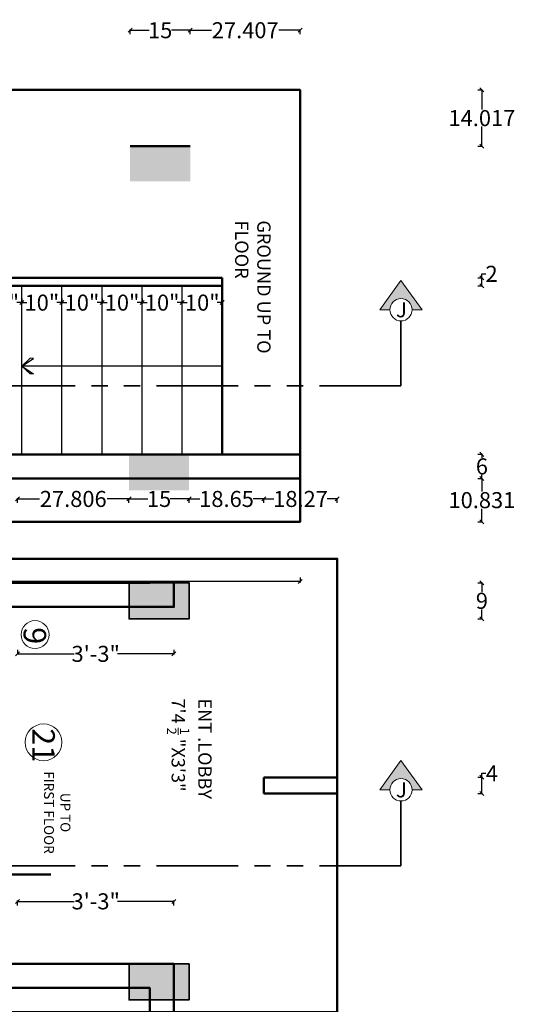
# Model space of a CAD drawing. Units: inches. Extents: x -60 to 284, y -245 to 257.
# Tile 10 of 10: x 160 to 284, y 12 to 257. Entities that reach past the tile are written whole.
import ezdxf

# ---------------------------------------------------------------- set-up
doc = ezdxf.new("R2010")
doc.units = ezdxf.units.IN
doc.header["$LTSCALE"] = 0.8
doc.header["$MEASUREMENT"] = 0
doc.linetypes.add('PHANTOM', pattern=[63.5, 31.75, -6.35, 6.35, -6.35, 6.35, -6.35])
for name, color, linetype, lineweight in [('A-ANNO-DIMS', 2, 'Continuous', 18), ('A-ANNO-SECT', 1, 'PHANTOM', 35), ('A-ANNO-SYMB', 3, 'Continuous', 18), ('A-ANNO-TEXT', 3, 'Continuous', 18), ('A-ANNO-TTLB', 7, 'Continuous', 50), ('A-COLS', 1, 'Continuous', 35), ('A-FLOR-STRS', 4, 'Continuous', 25), ('A-WALL', 7, 'Continuous', 50)]:
    doc.layers.add(name, color=color, linetype=linetype, lineweight=lineweight)
doc.styles.get("Standard").update_dxf_attribs({"font": 'arial.ttf'})
doc.dimstyles.get("Standard").update_dxf_attribs({"dimtxt": 4, "dimasz": 1, "dimexe": 0.18, "dimexo": 0.0625, "dimgap": 0.09, "dimtad": 0, "dimtih": 1, "dimtoh": 1, "dimzin": 0, "dimdsep": 46, "dimlunit": 4, "dimtxsty": 'Standard', "dimblk": 'OBLIQUE', "dimcen": 0.09, "dimadec": 0, "dimazin": 0, "dimtfac": 1, "dimtofl": 0, "dimtmove": 0, "dimatfit": 3, "dimfxl": 1, "dimfxlon": 1, "dimtolj": 1, "dimtzin": 0, "dimarcsym": 0})

# ---------------------------------------------------------------- blocks, each defined once
blk = doc.blocks.new('_Oblique')
at = {"color": 0, "linetype": 'ByBlock', "lineweight": -2}
blk.add_line((-0.5, -0.5), (0.5, 0.5), dxfattribs=at)
blk = doc.blocks.new('*D22')
at = {"layer": 'A-ANNO-DIMS', "color": 0, "lineweight": -2, "ltscale": 0.8, "transparency": 16777216}
for p, q in [((159.94, 36.25), (159.94, 37.43)), ((159.94, 37.25), (174.03, 37.25)), ((198.94, 37.25), (184.84, 37.25)), ((198.94, 36.25), (198.94, 37.43))]:
    blk.add_line(p, q, dxfattribs=at)
at = {"layer": 'Defpoints', "color": 0, "ltscale": 0.8, "transparency": 16777216}
for p in [(198.94, 37.25), (159.94, 21.67), (198.94, 21.67)]:
    blk.add_point(p, dxfattribs=at)
at = {"layer": 'A-ANNO-DIMS', "color": 0, "lineweight": -2, "ltscale": 0.8, "transparency": 16777216, "rotation": 180}
blk.add_blockref('_Oblique', (159.94, 37.25), dxfattribs=at)
at = {"layer": 'A-ANNO-DIMS', "color": 0, "lineweight": -2, "ltscale": 0.8, "transparency": 16777216}
blk.add_blockref('_Oblique', (198.94, 37.25), dxfattribs=at)
at = {"layer": 'A-ANNO-DIMS', "color": 0, "ltscale": 0.8, "transparency": 16777216, "insert": (179.44, 37.25), "char_height": 4, "attachment_point": 5}
blk.add_mtext('\\A1;3\'-3"', dxfattribs=at)
blk = doc.blocks.new('*D23')
at = {"layer": 'A-ANNO-DIMS', "color": 0, "lineweight": -2, "ltscale": 0.8, "transparency": 16777216}
for p, q in [((159.94, 99.95), (159.94, 98.77)), ((159.94, 98.95), (174.03, 98.95)), ((198.94, 98.95), (184.84, 98.95)), ((198.94, 99.95), (198.94, 98.77))]:
    blk.add_line(p, q, dxfattribs=at)
at = {"layer": 'Defpoints', "color": 0, "ltscale": 0.8, "transparency": 16777216}
for p in [(159.94, 110.67), (198.94, 110.67), (198.94, 98.95)]:
    blk.add_point(p, dxfattribs=at)
at = {"layer": 'A-ANNO-DIMS', "color": 0, "lineweight": -2, "ltscale": 0.8, "transparency": 16777216, "rotation": 180}
blk.add_blockref('_Oblique', (159.94, 98.95), dxfattribs=at)
at = {"layer": 'A-ANNO-DIMS', "color": 0, "lineweight": -2, "ltscale": 0.8, "transparency": 16777216}
blk.add_blockref('_Oblique', (198.94, 98.95), dxfattribs=at)
at = {"layer": 'A-ANNO-DIMS', "color": 0, "ltscale": 0.8, "transparency": 16777216, "insert": (179.44, 98.95), "char_height": 4, "attachment_point": 5}
blk.add_mtext('\\A1;3\'-3"', dxfattribs=at)
blk = doc.blocks.new('*D26')
at = {"layer": 'A-ANNO-DIMS', "color": 0, "lineweight": -2, "ltscale": 0.8, "transparency": 16777216}
for p, q in [((201.01, 186.51), (201.01, 186.69)), ((211.01, 186.51), (211.01, 186.69)), ((201.01, 186.51), (202.26, 186.51)), ((211.01, 186.51), (209.77, 186.51))]:
    blk.add_line(p, q, dxfattribs=at)
at = {"layer": 'Defpoints', "color": 0, "ltscale": 0.8, "transparency": 16777216}
for p in [(201.01, 186.51), (201.01, 186.51), (211.01, 186.51)]:
    blk.add_point(p, dxfattribs=at)
at = {"layer": 'A-ANNO-DIMS', "color": 0, "lineweight": -2, "ltscale": 0.8, "transparency": 16777216, "rotation": 180}
blk.add_blockref('_Oblique', (201.01, 186.51), dxfattribs=at)
at = {"layer": 'A-ANNO-DIMS', "color": 0, "lineweight": -2, "ltscale": 0.8, "transparency": 16777216}
blk.add_blockref('_Oblique', (211.01, 186.51), dxfattribs=at)
at = {"layer": 'A-ANNO-DIMS', "color": 0, "ltscale": 0.8, "transparency": 16777216, "insert": (206.01, 186.51), "char_height": 4, "attachment_point": 5}
blk.add_mtext('\\A1;10"', dxfattribs=at)
blk = doc.blocks.new('*D27')
at = {"layer": 'A-ANNO-DIMS', "color": 0, "lineweight": -2, "ltscale": 0.8, "transparency": 16777216}
for p, q in [((191.01, 186.51), (191.01, 186.69)), ((201.01, 186.51), (201.01, 186.69)), ((191.01, 186.51), (192.26, 186.51)), ((201.01, 186.51), (199.77, 186.51))]:
    blk.add_line(p, q, dxfattribs=at)
at = {"layer": 'Defpoints', "color": 0, "ltscale": 0.8, "transparency": 16777216}
for p in [(191.01, 186.51), (191.01, 186.51), (201.01, 186.51)]:
    blk.add_point(p, dxfattribs=at)
at = {"layer": 'A-ANNO-DIMS', "color": 0, "lineweight": -2, "ltscale": 0.8, "transparency": 16777216, "rotation": 180}
blk.add_blockref('_Oblique', (191.01, 186.51), dxfattribs=at)
at = {"layer": 'A-ANNO-DIMS', "color": 0, "lineweight": -2, "ltscale": 0.8, "transparency": 16777216}
blk.add_blockref('_Oblique', (201.01, 186.51), dxfattribs=at)
at = {"layer": 'A-ANNO-DIMS', "color": 0, "ltscale": 0.8, "transparency": 16777216, "insert": (196.01, 186.51), "char_height": 4, "attachment_point": 5}
blk.add_mtext('\\A1;10"', dxfattribs=at)
blk = doc.blocks.new('*D28')
at = {"layer": 'A-ANNO-DIMS', "color": 0, "lineweight": -2, "ltscale": 0.8, "transparency": 16777216}
for p, q in [((181.01, 187.51), (181.01, 186.33)), ((191.01, 187.51), (191.01, 186.33)), ((181.01, 186.51), (182.26, 186.51)), ((191.01, 186.51), (189.77, 186.51))]:
    blk.add_line(p, q, dxfattribs=at)
at = {"layer": 'Defpoints', "color": 0, "ltscale": 0.8, "transparency": 16777216}
for p in [(181.01, 187.62), (191.01, 187.62), (191.01, 186.51)]:
    blk.add_point(p, dxfattribs=at)
at = {"layer": 'A-ANNO-DIMS', "color": 0, "lineweight": -2, "ltscale": 0.8, "transparency": 16777216, "rotation": 180}
blk.add_blockref('_Oblique', (181.01, 186.51), dxfattribs=at)
at = {"layer": 'A-ANNO-DIMS', "color": 0, "lineweight": -2, "ltscale": 0.8, "transparency": 16777216}
blk.add_blockref('_Oblique', (191.01, 186.51), dxfattribs=at)
at = {"layer": 'A-ANNO-DIMS', "color": 0, "ltscale": 0.8, "transparency": 16777216, "insert": (186.01, 186.51), "char_height": 4, "attachment_point": 5}
blk.add_mtext('\\A1;10"', dxfattribs=at)
blk = doc.blocks.new('*D29')
at = {"layer": 'A-ANNO-DIMS', "color": 0, "lineweight": -2, "ltscale": 0.8, "transparency": 16777216}
for p, q in [((171.01, 187.47), (171.01, 186.33)), ((181.01, 187.51), (181.01, 186.33)), ((171.01, 186.51), (172.26, 186.51)), ((181.01, 186.51), (179.77, 186.51))]:
    blk.add_line(p, q, dxfattribs=at)
at = {"layer": 'Defpoints', "color": 0, "ltscale": 0.8, "transparency": 16777216}
for p in [(171.01, 187.53), (181.01, 187.62), (181.01, 186.51)]:
    blk.add_point(p, dxfattribs=at)
at = {"layer": 'A-ANNO-DIMS', "color": 0, "lineweight": -2, "ltscale": 0.8, "transparency": 16777216, "rotation": 180}
blk.add_blockref('_Oblique', (171.01, 186.51), dxfattribs=at)
at = {"layer": 'A-ANNO-DIMS', "color": 0, "lineweight": -2, "ltscale": 0.8, "transparency": 16777216}
blk.add_blockref('_Oblique', (181.01, 186.51), dxfattribs=at)
at = {"layer": 'A-ANNO-DIMS', "color": 0, "ltscale": 0.8, "transparency": 16777216, "insert": (176.01, 186.51), "char_height": 4, "attachment_point": 5}
blk.add_mtext('\\A1;10"', dxfattribs=at)
blk = doc.blocks.new('*D30')
at = {"layer": 'A-ANNO-DIMS', "color": 0, "lineweight": -2, "ltscale": 0.8, "transparency": 16777216}
for p, q in [((161.01, 187.51), (161.01, 186.33)), ((171.01, 187.51), (171.01, 186.33)), ((161.01, 186.51), (162.26, 186.51)), ((171.01, 186.51), (169.77, 186.51))]:
    blk.add_line(p, q, dxfattribs=at)
at = {"layer": 'Defpoints', "color": 0, "ltscale": 0.8, "transparency": 16777216}
for p in [(161.01, 187.69), (171.01, 187.69), (171.01, 186.51)]:
    blk.add_point(p, dxfattribs=at)
at = {"layer": 'A-ANNO-DIMS', "color": 0, "lineweight": -2, "ltscale": 0.8, "transparency": 16777216, "rotation": 180}
blk.add_blockref('_Oblique', (161.01, 186.51), dxfattribs=at)
at = {"layer": 'A-ANNO-DIMS', "color": 0, "lineweight": -2, "ltscale": 0.8, "transparency": 16777216}
blk.add_blockref('_Oblique', (171.01, 186.51), dxfattribs=at)
at = {"layer": 'A-ANNO-DIMS', "color": 0, "ltscale": 0.8, "transparency": 16777216, "insert": (166.01, 186.51), "char_height": 4, "attachment_point": 5}
blk.add_mtext('\\A1;10"', dxfattribs=at)
blk = doc.blocks.new('*D31')
at = {"layer": 'A-ANNO-DIMS', "color": 0, "lineweight": -2, "ltscale": 0.8, "transparency": 16777216}
for p, q in [((151.01, 187.51), (151.01, 186.33)), ((161.01, 187.51), (161.01, 186.33)), ((151.01, 186.51), (152.26, 186.51)), ((161.01, 186.51), (159.77, 186.51))]:
    blk.add_line(p, q, dxfattribs=at)
at = {"layer": 'Defpoints', "color": 0, "ltscale": 0.8, "transparency": 16777216}
for p in [(151.01, 187.73), (161.01, 187.73), (161.01, 186.51)]:
    blk.add_point(p, dxfattribs=at)
at = {"layer": 'A-ANNO-DIMS', "color": 0, "lineweight": -2, "ltscale": 0.8, "transparency": 16777216, "rotation": 180}
blk.add_blockref('_Oblique', (151.01, 186.51), dxfattribs=at)
at = {"layer": 'A-ANNO-DIMS', "color": 0, "lineweight": -2, "ltscale": 0.8, "transparency": 16777216}
blk.add_blockref('_Oblique', (161.01, 186.51), dxfattribs=at)
at = {"layer": 'A-ANNO-DIMS', "color": 0, "ltscale": 0.8, "transparency": 16777216, "insert": (156.01, 186.51), "char_height": 4, "attachment_point": 5}
blk.add_mtext('\\A1;10"', dxfattribs=at)
blk = doc.blocks.new('SECTION-MARK')
at = {"ltscale": 0.8}
for p, q in [((0, 2.79), (5.28, 10.08)), ((10.57, 2.79), (5.28, 10.08)), ((2.5, 2.79), (0, 2.79)), ((8.07, 2.79), (10.57, 2.79))]:
    blk.add_line(p, q, dxfattribs=at)
blk.add_circle((5.28, 2.79), 2.79, dxfattribs=at)
blk = doc.blocks.new('STAIR-ARROW')
at = {"ltscale": 0.8}
for p, q in [((2.04, 3.88), (0, 1.94)), ((0, 1.94), (2.88, 3.86)), ((2.88, 3.86), (2.04, 3.88)), ((50, 1.94), (0, 1.94)), ((0, 1.94), (2.88, 0.03)), ((2.04, 0), (0, 1.94)), ((2.88, 0.03), (2.04, 0))]:
    blk.add_line(p, q, dxfattribs=at)
blk = doc.blocks.new('*D76')
at = {"layer": 'A-ANNO-DIMS', "color": 0, "lineweight": -2, "ltscale": 0.8, "transparency": 16777216}
for p, q in [((-0.88, 117.95), (-0.88, 116.77)), ((230.43, 117.95), (230.43, 116.77)), ((-0.88, 116.95), (107.9, 116.95)), ((230.43, 116.95), (121.65, 116.95))]:
    blk.add_line(p, q, dxfattribs=at)
at = {"layer": 'Defpoints', "color": 0, "ltscale": 0.8, "transparency": 16777216}
for p in [(-0.88, 131.85), (230.43, 131.85), (230.43, 116.95)]:
    blk.add_point(p, dxfattribs=at)
at = {"layer": 'A-ANNO-DIMS', "color": 0, "lineweight": -2, "ltscale": 0.8, "transparency": 16777216, "rotation": 180}
blk.add_blockref('_Oblique', (-0.88, 116.95), dxfattribs=at)
at = {"layer": 'A-ANNO-DIMS', "color": 0, "lineweight": -2, "ltscale": 0.8, "transparency": 16777216}
blk.add_blockref('_Oblique', (230.43, 116.95), dxfattribs=at)
at = {"layer": 'A-ANNO-DIMS', "color": 0, "ltscale": 0.8, "transparency": 16777216, "insert": (114.78, 116.95), "char_height": 4, "attachment_point": 5}
blk.add_mtext('\\A1;231.3', dxfattribs=at)
blk = doc.blocks.new('*D81')
at = {"layer": 'A-ANNO-DIMS', "color": 0, "lineweight": -2, "ltscale": 0.8, "transparency": 16777216}
for p, q in [((188.02, 253.42), (188.02, 254.6)), ((188.02, 254.42), (192.74, 254.42)), ((203.02, 254.42), (198.3, 254.42)), ((203.02, 253.42), (203.02, 254.6))]:
    blk.add_line(p, q, dxfattribs=at)
at = {"layer": 'Defpoints', "color": 0, "ltscale": 0.8, "transparency": 16777216}
for p in [(203.02, 254.42), (188.02, 225.5), (203.02, 225.5)]:
    blk.add_point(p, dxfattribs=at)
at = {"layer": 'A-ANNO-DIMS', "color": 0, "lineweight": -2, "ltscale": 0.8, "transparency": 16777216, "rotation": 180}
blk.add_blockref('_Oblique', (188.02, 254.42), dxfattribs=at)
at = {"layer": 'A-ANNO-DIMS', "color": 0, "lineweight": -2, "ltscale": 0.8, "transparency": 16777216}
blk.add_blockref('_Oblique', (203.02, 254.42), dxfattribs=at)
at = {"layer": 'A-ANNO-DIMS', "color": 0, "ltscale": 0.8, "transparency": 16777216, "insert": (195.52, 254.42), "char_height": 4, "attachment_point": 5}
blk.add_mtext('\\A1;15', dxfattribs=at)
blk = doc.blocks.new('*D82')
at = {"layer": 'A-ANNO-DIMS', "color": 0, "lineweight": -2, "ltscale": 0.8, "transparency": 16777216}
for p, q in [((203.02, 253.42), (203.02, 254.6)), ((203.02, 254.42), (208.3, 254.42)), ((230.43, 254.42), (225.15, 254.42)), ((230.43, 253.42), (230.43, 254.6))]:
    blk.add_line(p, q, dxfattribs=at)
at = {"layer": 'Defpoints', "color": 0, "ltscale": 0.8, "transparency": 16777216}
for p in [(230.43, 254.42), (230.43, 239.52), (203.02, 225.5)]:
    blk.add_point(p, dxfattribs=at)
at = {"layer": 'A-ANNO-DIMS', "color": 0, "lineweight": -2, "ltscale": 0.8, "transparency": 16777216, "rotation": 180}
blk.add_blockref('_Oblique', (203.02, 254.42), dxfattribs=at)
at = {"layer": 'A-ANNO-DIMS', "color": 0, "lineweight": -2, "ltscale": 0.8, "transparency": 16777216}
blk.add_blockref('_Oblique', (230.43, 254.42), dxfattribs=at)
at = {"layer": 'A-ANNO-DIMS', "color": 0, "ltscale": 0.8, "transparency": 16777216, "insert": (216.73, 254.42), "char_height": 4, "attachment_point": 5}
blk.add_mtext('\\A1;27.407', dxfattribs=at)
blk = doc.blocks.new('*D83')
at = {"layer": 'A-ANNO-DIMS', "color": 0, "lineweight": -2, "ltscale": 0.8, "transparency": 16777216}
for p, q in [((274.76, 148.69), (275.94, 148.69)), ((275.76, 148.69), (275.76, 147.82)), ((274.76, 142.69), (275.94, 142.69)), ((275.76, 142.69), (275.76, 143.55))]:
    blk.add_line(p, q, dxfattribs=at)
at = {"layer": 'Defpoints', "color": 0, "ltscale": 0.8, "transparency": 16777216}
for p in [(230.43, 148.69), (275.76, 148.69), (230.43, 142.69)]:
    blk.add_point(p, dxfattribs=at)
at = {"layer": 'A-ANNO-DIMS', "color": 0, "lineweight": -2, "ltscale": 0.8, "transparency": 16777216}
for p, rotation in [((275.76, 148.69), 90), ((275.76, 142.69), 270)]:
    blk.add_blockref('_Oblique', p, dxfattribs=dict(at, rotation=rotation))
at = {"layer": 'A-ANNO-DIMS', "color": 0, "ltscale": 0.8, "transparency": 16777216, "insert": (275.76, 145.69), "char_height": 4, "attachment_point": 5}
blk.add_mtext('\\A1;6', dxfattribs=at)
blk = doc.blocks.new('*D84')
at = {"layer": 'A-ANNO-DIMS', "color": 0, "lineweight": -2, "ltscale": 0.8, "transparency": 16777216}
for p, q in [((274.76, 142.69), (275.94, 142.69)), ((275.76, 142.69), (275.76, 139.4)), ((275.76, 131.85), (275.76, 135.14)), ((274.76, 131.85), (275.94, 131.85))]:
    blk.add_line(p, q, dxfattribs=at)
at = {"layer": 'Defpoints', "color": 0, "ltscale": 0.8, "transparency": 16777216}
for p in [(230.43, 142.69), (275.76, 142.69), (230.43, 131.85)]:
    blk.add_point(p, dxfattribs=at)
at = {"layer": 'A-ANNO-DIMS', "color": 0, "lineweight": -2, "ltscale": 0.8, "transparency": 16777216}
for p, rotation in [((275.76, 142.69), 90), ((275.76, 131.85), 270)]:
    blk.add_blockref('_Oblique', p, dxfattribs=dict(at, rotation=rotation))
at = {"layer": 'A-ANNO-DIMS', "color": 0, "ltscale": 0.8, "transparency": 16777216, "insert": (275.76, 137.27), "char_height": 4, "attachment_point": 5}
blk.add_mtext('\\A1;10.831', dxfattribs=at)
blk = doc.blocks.new('*D85')
at = {"layer": 'A-ANNO-DIMS', "color": 0, "lineweight": -2, "ltscale": 0.8, "transparency": 16777216}
for p, q in [((274.76, 192.69), (275.94, 192.69)), ((275.76, 192.69), (275.76, 193.69)), ((275.76, 193.69), (276.76, 193.69)), ((275.76, 190.69), (275.76, 192.69)), ((274.76, 190.69), (275.94, 190.69))]:
    blk.add_line(p, q, dxfattribs=at)
at = {"layer": 'Defpoints', "color": 0, "ltscale": 0.8, "transparency": 16777216}
for p in [(211.01, 192.69), (275.76, 192.69), (211.01, 190.69)]:
    blk.add_point(p, dxfattribs=at)
at = {"layer": 'A-ANNO-DIMS', "color": 0, "lineweight": -2, "ltscale": 0.8, "transparency": 16777216}
for p, rotation in [((275.76, 192.69), 90), ((275.76, 190.69), 270)]:
    blk.add_blockref('_Oblique', p, dxfattribs=dict(at, rotation=rotation))
at = {"layer": 'A-ANNO-DIMS', "color": 0, "ltscale": 0.8, "transparency": 16777216, "insert": (278.18, 193.69), "char_height": 4, "attachment_point": 5}
blk.add_mtext('\\A1;2', dxfattribs=at)
blk = doc.blocks.new('*D86')
at = {"layer": 'A-ANNO-DIMS', "color": 0, "lineweight": -2, "ltscale": 0.8, "transparency": 16777216}
for p, q in [((274.76, 239.52), (275.94, 239.52)), ((275.76, 239.52), (275.76, 234.64)), ((275.76, 225.5), (275.76, 230.38)), ((274.76, 225.5), (275.94, 225.5))]:
    blk.add_line(p, q, dxfattribs=at)
at = {"layer": 'Defpoints', "color": 0, "ltscale": 0.8, "transparency": 16777216}
for p in [(230.43, 239.52), (275.76, 239.52), (203.02, 225.5)]:
    blk.add_point(p, dxfattribs=at)
at = {"layer": 'A-ANNO-DIMS', "color": 0, "lineweight": -2, "ltscale": 0.8, "transparency": 16777216}
for p, rotation in [((275.76, 239.52), 90), ((275.76, 225.5), 270)]:
    blk.add_blockref('_Oblique', p, dxfattribs=dict(at, rotation=rotation))
at = {"layer": 'A-ANNO-DIMS', "color": 0, "ltscale": 0.8, "transparency": 16777216, "insert": (275.76, 232.51), "char_height": 4, "attachment_point": 5}
blk.add_mtext('\\A1;14.017', dxfattribs=at)
blk = doc.blocks.new('*D95')
at = {"layer": 'A-ANNO-DIMS', "color": 0, "lineweight": -2, "ltscale": 0.8, "transparency": 16777216}
for p, q in [((159.94, 136.57), (159.94, 137.75)), ((159.94, 137.57), (165.41, 137.57)), ((187.74, 137.57), (182.26, 137.57)), ((187.74, 136.57), (187.74, 137.75))]:
    blk.add_line(p, q, dxfattribs=at)
at = {"layer": 'Defpoints', "color": 0, "ltscale": 0.8, "transparency": 16777216}
for p in [(187.74, 137.57), (159.94, 110.67), (187.74, 107.67)]:
    blk.add_point(p, dxfattribs=at)
at = {"layer": 'A-ANNO-DIMS', "color": 0, "lineweight": -2, "ltscale": 0.8, "transparency": 16777216, "rotation": 180}
blk.add_blockref('_Oblique', (159.94, 137.57), dxfattribs=at)
at = {"layer": 'A-ANNO-DIMS', "color": 0, "lineweight": -2, "ltscale": 0.8, "transparency": 16777216}
blk.add_blockref('_Oblique', (187.74, 137.57), dxfattribs=at)
at = {"layer": 'A-ANNO-DIMS', "color": 0, "ltscale": 0.8, "transparency": 16777216, "insert": (173.84, 137.57), "char_height": 4, "attachment_point": 5}
blk.add_mtext('\\A1;27.806', dxfattribs=at)
blk = doc.blocks.new('*D96')
at = {"layer": 'A-ANNO-DIMS', "color": 0, "lineweight": -2, "ltscale": 0.8, "transparency": 16777216}
for p, q in [((187.74, 136.57), (187.74, 137.75)), ((187.74, 137.57), (192.46, 137.57)), ((202.74, 137.57), (198.02, 137.57)), ((202.74, 136.57), (202.74, 137.75))]:
    blk.add_line(p, q, dxfattribs=at)
at = {"layer": 'Defpoints', "color": 0, "ltscale": 0.8, "transparency": 16777216}
for p in [(202.74, 137.57), (187.74, 107.67), (202.74, 107.67)]:
    blk.add_point(p, dxfattribs=at)
at = {"layer": 'A-ANNO-DIMS', "color": 0, "lineweight": -2, "ltscale": 0.8, "transparency": 16777216, "rotation": 180}
blk.add_blockref('_Oblique', (187.74, 137.57), dxfattribs=at)
at = {"layer": 'A-ANNO-DIMS', "color": 0, "lineweight": -2, "ltscale": 0.8, "transparency": 16777216}
blk.add_blockref('_Oblique', (202.74, 137.57), dxfattribs=at)
at = {"layer": 'A-ANNO-DIMS', "color": 0, "ltscale": 0.8, "transparency": 16777216, "insert": (195.24, 137.57), "char_height": 4, "attachment_point": 5}
blk.add_mtext('\\A1;15', dxfattribs=at)
blk = doc.blocks.new('*D97')
at = {"layer": 'A-ANNO-DIMS', "color": 0, "lineweight": -2, "ltscale": 0.8, "transparency": 16777216}
for p, q in [((202.74, 136.57), (202.74, 137.75)), ((202.74, 137.57), (205.4, 137.57)), ((221.39, 137.57), (218.73, 137.57)), ((221.39, 136.57), (221.39, 137.75))]:
    blk.add_line(p, q, dxfattribs=at)
at = {"layer": 'Defpoints', "color": 0, "ltscale": 0.8, "transparency": 16777216}
for p in [(221.39, 137.57), (202.74, 107.67), (221.39, 68.17)]:
    blk.add_point(p, dxfattribs=at)
at = {"layer": 'A-ANNO-DIMS', "color": 0, "lineweight": -2, "ltscale": 0.8, "transparency": 16777216, "rotation": 180}
blk.add_blockref('_Oblique', (202.74, 137.57), dxfattribs=at)
at = {"layer": 'A-ANNO-DIMS', "color": 0, "lineweight": -2, "ltscale": 0.8, "transparency": 16777216}
blk.add_blockref('_Oblique', (221.39, 137.57), dxfattribs=at)
at = {"layer": 'A-ANNO-DIMS', "color": 0, "ltscale": 0.8, "transparency": 16777216, "insert": (212.07, 137.57), "char_height": 4, "attachment_point": 5}
blk.add_mtext('\\A1;18.65', dxfattribs=at)
blk = doc.blocks.new('*D98')
at = {"layer": 'A-ANNO-DIMS', "color": 0, "lineweight": -2, "ltscale": 0.8, "transparency": 16777216}
for p, q in [((221.39, 136.57), (221.39, 137.75)), ((221.39, 137.57), (223.88, 137.57)), ((239.66, 137.57), (237.18, 137.57)), ((239.66, 136.57), (239.66, 137.75))]:
    blk.add_line(p, q, dxfattribs=at)
at = {"layer": 'Defpoints', "color": 0, "ltscale": 0.8, "transparency": 16777216}
for p in [(239.66, 137.57), (239.66, 122.67), (221.39, 68.17)]:
    blk.add_point(p, dxfattribs=at)
at = {"layer": 'A-ANNO-DIMS', "color": 0, "lineweight": -2, "ltscale": 0.8, "transparency": 16777216, "rotation": 180}
blk.add_blockref('_Oblique', (221.39, 137.57), dxfattribs=at)
at = {"layer": 'A-ANNO-DIMS', "color": 0, "lineweight": -2, "ltscale": 0.8, "transparency": 16777216}
blk.add_blockref('_Oblique', (239.66, 137.57), dxfattribs=at)
at = {"layer": 'A-ANNO-DIMS', "color": 0, "ltscale": 0.8, "transparency": 16777216, "insert": (230.53, 137.57), "char_height": 4, "attachment_point": 5}
blk.add_mtext('\\A1;18.27', dxfattribs=at)
blk = doc.blocks.new('*D103')
at = {"layer": 'A-ANNO-DIMS', "color": 0, "lineweight": -2, "ltscale": 0.8, "transparency": 16777216}
for p, q in [((274.76, 116.67), (275.94, 116.67)), ((275.76, 116.67), (275.76, 114.3)), ((275.76, 107.67), (275.76, 110.03)), ((274.76, 107.67), (275.94, 107.67))]:
    blk.add_line(p, q, dxfattribs=at)
at = {"layer": 'Defpoints', "color": 0, "ltscale": 0.8, "transparency": 16777216}
for p in [(202.74, 116.67), (275.76, 116.67), (202.74, 107.67)]:
    blk.add_point(p, dxfattribs=at)
at = {"layer": 'A-ANNO-DIMS', "color": 0, "lineweight": -2, "ltscale": 0.8, "transparency": 16777216}
for p, rotation in [((275.76, 116.67), 90), ((275.76, 107.67), 270)]:
    blk.add_blockref('_Oblique', p, dxfattribs=dict(at, rotation=rotation))
at = {"layer": 'A-ANNO-DIMS', "color": 0, "ltscale": 0.8, "transparency": 16777216, "insert": (275.76, 112.17), "char_height": 4, "attachment_point": 5}
blk.add_mtext('\\A1;9', dxfattribs=at)
blk = doc.blocks.new('*D104')
at = {"layer": 'A-ANNO-DIMS', "color": 0, "lineweight": -2, "ltscale": 0.8, "transparency": 16777216}
for p, q in [((275.76, 68.17), (275.76, 69.17)), ((275.76, 69.17), (276.76, 69.17)), ((274.76, 68.17), (275.94, 68.17)), ((275.76, 64.17), (275.76, 68.17)), ((274.76, 64.17), (275.94, 64.17))]:
    blk.add_line(p, q, dxfattribs=at)
at = {"layer": 'Defpoints', "color": 0, "ltscale": 0.8, "transparency": 16777216}
for p in [(221.39, 68.17), (275.76, 68.17), (221.39, 64.17)]:
    blk.add_point(p, dxfattribs=at)
at = {"layer": 'A-ANNO-DIMS', "color": 0, "lineweight": -2, "ltscale": 0.8, "transparency": 16777216}
for p, rotation in [((275.76, 68.17), 90), ((275.76, 64.17), 270)]:
    blk.add_blockref('_Oblique', p, dxfattribs=dict(at, rotation=rotation))
at = {"layer": 'A-ANNO-DIMS', "color": 0, "ltscale": 0.8, "transparency": 16777216, "insert": (278.24, 69.17), "char_height": 4, "attachment_point": 5}
blk.add_mtext('\\A1;4', dxfattribs=at)

msp = doc.modelspace()

# ---------------------------------------------------------------- hatches: boundary and pattern name
at = {"layer": 'A-ANNO-SYMB', "ltscale": 0.8}
h = msp.add_hatch(color=256, dxfattribs=at)
h.dxf.hatch_style = 1
h.paths.add_polyline_path([(250.2979, 184.7402), (252.7949, 184.7402, -1), (258.3665, 184.7402), (260.8636, 184.7402), (255.5807, 192.0356)])
h = msp.add_hatch(color=256, dxfattribs=at)
h.dxf.hatch_style = 1
h.paths.add_polyline_path([(255.5807, 72.3512), (250.2979, 65.0558), (252.7949, 65.0558, -1), (258.3665, 65.0558), (260.8636, 65.0558)])
at = {"layer": 'A-COLS', "ltscale": 0.8}
h = msp.add_hatch(color=256, dxfattribs=at)
h.dxf.hatch_style = 1
h.paths.add_polyline_path([(203.0229, 225.7452), (188.0229, 225.7452), (188.0229, 216.7452), (203.0229, 216.7452)])
h = msp.add_hatch(color=256, dxfattribs=at)
h.dxf.hatch_style = 1
h.paths.add_polyline_path([(202.7426, 148.6856), (187.7426, 148.6856), (187.7426, 139.6856), (202.7426, 139.6856)])
h = msp.add_hatch(color=256, dxfattribs=at)
h.dxf.hatch_style = 1
h.paths.add_polyline_path([(202.7426, 116.666), (187.7426, 116.666), (187.7426, 107.666), (202.7426, 107.666)])
h = msp.add_hatch(color=256, dxfattribs=at)
h.dxf.hatch_style = 1
h.paths.add_polyline_path([(202.7426, 21.666), (187.7426, 21.666), (187.7426, 12.666), (202.7426, 12.666)])

# ---------------------------------------------------------------- linework, layer by layer
at = {"layer": 'A-ANNO-SECT', "ltscale": 0.8}
for p, q in [((255.5807, 181.9544), (255.5807, 165.8004)), ((255.5807, 165.8004), (-23.5489, 165.8004)), ((255.5807, 62.27), (255.5807, 46.116)), ((255.5807, 46.116), (-23.5489, 46.116))]:
    msp.add_line(p, q, dxfattribs=at)
at = {"layer": 'A-ANNO-SYMB', "ltscale": 0.8}
for centre, radius in [((164.3195, 103.7534), 3.4808), ((166.4188, 76.8954), 4.5856)]:
    msp.add_circle(centre, radius, dxfattribs=at)
at = {"layer": 'A-ANNO-TTLB', "ltscale": 0.8}
for points in [[(-0.8787, 239.5184), (230.4297, 239.5184), (230.4297, 131.8542), (-0.8787, 131.8542)], [(0.0867, 122.666), (239.6639, 122.666), (239.6639, 9.666), (0.0867, 9.666)]]:
    msp.add_lwpolyline(points, close=True, dxfattribs=at)
at = {"layer": 'A-COLS', "ltscale": 0.8}
for points in [[(187.7426, 116.666), (202.7426, 116.666), (202.7426, 107.666), (187.7426, 107.666)], [(187.7426, 21.666), (202.7426, 21.666), (202.7426, 12.666), (187.7426, 12.666)]]:
    msp.add_lwpolyline(points, close=True, dxfattribs=at)
at = {"layer": 'A-FLOR-STRS', "ltscale": 0.8}
for p, q in [((161.0139, 148.6856), (161.0139, 190.6856)), ((171.0139, 148.6856), (171.0139, 190.6856)), ((181.0139, 148.6856), (181.0139, 190.6856)), ((191.0139, 148.6856), (191.0139, 190.6856)), ((201.0139, 148.6856), (201.0139, 190.6856))]:
    msp.add_line(p, q, dxfattribs=at)
at = {"layer": 'A-WALL', "ltscale": 0.8}
for p, q in [((203.0229, 225.5014), (188.0229, 225.5014)), ((67.0139, 192.6856), (211.0139, 192.6856)), ((211.0139, 148.6856), (211.0139, 192.6856)), ((67.0139, 190.6856), (211.0139, 190.6856)), ((82.0139, 148.6856), (230.4297, 148.6856)), ((82.0139, 142.6856), (230.4297, 142.6856)), ((239.6639, 68.166), (221.3929, 68.166)), ((221.3929, 64.166), (221.3929, 68.166)), ((239.6639, 64.166), (221.3929, 64.166)), ((168.271, 43.916), (43.6123, 43.916))]:
    msp.add_line(p, q, dxfattribs=at)
at = {"layer": 'A-WALL'}
for points in [[(198.9361, 116.666), (198.9361, 110.666), (159.9361, 110.666), (79.9361, 110.666), (37.9361, 110.666), (27.9361, 110.666), (27.9361, 122.666)], [(192.9361, 116.666), (159.9361, 116.666), (79.9361, 116.666), (37.9361, 116.666), (33.9361, 116.666), (33.9361, 122.666)], [(198.9361, 9.666), (198.9361, 21.666), (159.9361, 21.666), (79.9361, 21.666), (37.9361, 21.666), (27.9361, 21.666), (27.9361, 9.666)], [(192.9361, 9.666), (192.9361, 15.666), (159.9361, 15.666), (79.9361, 15.666), (37.9361, 15.666), (33.9361, 15.666), (33.9361, 9.666)]]:
    msp.add_lwpolyline(points, dxfattribs=at)

# ---------------------------------------------------------------- block references
at = {"layer": 'A-ANNO-SYMB'}
for p in [(250.298, 181.9544), (250.298, 62.27)]:
    msp.add_blockref('SECTION-MARK', p, dxfattribs=at)
at = {"layer": 'A-FLOR-STRS'}
msp.add_blockref('STAIR-ARROW', (161.014, 168.744), dxfattribs=at)

# ---------------------------------------------------------------- texts
at = {"layer": 'A-ANNO-TEXT', "ltscale": 0.8, "rotation": 270}
for s, width, gutter_width, insert, char_height, attachment_point in [('\\A1;GROUND UP TO \\PFLOOR', 69.138891, 0.3685, (223.0466, 207.0118), 3.316205, 1), ('9', 28.020867, 2.8021, (161.4581, 105.596), 5.6042, 7), ('\\A1;ENT .LOBBY\\P7\'4 {\\H0.7x;\\S1/2;} "X3\'3"', 69.138891, 0.3685, (208.3424, 87.8373), 3.316205, 1), ('21', 28.020867, 2.8021, (169.2324, 80.4161), 5.60417, 1), ('\\pxqc;UP TO\\PFIRST FLOOR', 51.337432, 0.2736, (173.1145, 85.0647), 2.462369, 1)]:
    msp.add_mtext_dynamic_manual_height_columns(s, width=width, gutter_width=gutter_width, heights=[0], dxfattribs=dict(at, insert=insert, char_height=char_height, attachment_point=attachment_point))
at = {"layer": 'A-ANNO-TEXT', "ltscale": 0.8, "char_height": 3.7545, "attachment_point": 1}
for insert in [(254.31, 186.6092), (254.31, 66.9248)]:
    msp.add_mtext_dynamic_manual_height_columns('J', width=2.355391, gutter_width=0.4172, heights=[0], dxfattribs=dict(at, insert=insert))

# ---------------------------------------------------------------- dimensions: what is measured, and where the dimension line sits
at = {"layer": 'A-ANNO-DIMS', "ltscale": 0.8}
for base, p1, p2, override, picture, middle in [((203.0229, 254.4184), (188.0229, 225.5014), (203.0229, 225.5014), {"dimdec": 0, "dimlfac": 1, "dimrnd": 0, "dimzin": 0, "dimdsep": 46, "dimlunit": 2}, '*D81', (195.5229, 254.4184)), ((230.4297, 254.4184), (203.0229, 225.5014), (230.4297, 239.5184), {"dimdec": 3, "dimlfac": 1, "dimrnd": 0, "dimzin": 0, "dimdsep": 46, "dimlunit": 2}, '*D82', (216.7263, 254.4184)), ((161.0139, 186.5084), (151.0139, 187.7334), (161.0139, 187.7334), {"dimclrd": 0, "dimclre": 0, "dimclrt": 0}, '*D31', (156.0139, 186.5084)), ((171.0139, 186.5084), (161.0139, 187.6929), (171.0139, 187.6929), {"dimclrd": 0, "dimclre": 0, "dimclrt": 0}, '*D30', (166.0139, 186.5084)), ((181.0139, 186.5084), (171.0139, 187.5318), (181.0139, 187.62), {"dimclrd": 0, "dimclre": 0, "dimclrt": 0}, '*D29', (176.0139, 186.5084)), ((191.0139, 186.5084), (181.0139, 187.62), (191.0139, 187.62), {"dimclrd": 0, "dimclre": 0, "dimclrt": 0}, '*D28', (186.0139, 186.5084)), ((191.0139, 186.5084), (201.0139, 186.5084), (191.0139, 186.5084), {"dimclrd": 0, "dimclre": 0, "dimclrt": 0}, '*D27', (196.0139, 186.5084)), ((201.0139, 186.5084), (211.0139, 186.5084), (201.0139, 186.5084), {"dimclrd": 0, "dimclre": 0, "dimclrt": 0}, '*D26', (206.0139, 186.5084)), ((187.74258, 137.56605), (159.93611, 110.66605), (187.74258, 107.66605), {"dimdec": 3, "dimlfac": 1, "dimrnd": 0, "dimzin": 0, "dimdsep": 46, "dimlunit": 2}, '*D95', (173.83935, 137.56605)), ((202.7426, 137.566), (187.7426, 107.666), (202.7426, 107.666), {"dimdec": 0, "dimlfac": 1, "dimrnd": 0, "dimzin": 0, "dimdsep": 46, "dimlunit": 2}, '*D96', (195.2426, 137.566)), ((221.3929, 137.566), (202.7426, 107.666), (221.3929, 68.166), {"dimdec": 2, "dimlfac": 1, "dimrnd": 0, "dimzin": 0, "dimdsep": 46, "dimlunit": 2}, '*D97', (212.0677, 137.566)), ((239.6639, 137.566), (221.3929, 68.166), (239.6639, 122.666), {"dimdec": 2, "dimlfac": 1, "dimrnd": 0, "dimzin": 0, "dimdsep": 46, "dimlunit": 2}, '*D98', (230.5284, 137.566)), ((230.4297, 116.9542), (-0.8787, 131.8542), (230.4297, 131.8542), {"dimdec": 1, "dimlfac": 1, "dimrnd": 0, "dimzin": 0, "dimdsep": 46, "dimlunit": 2}, '*D76', (114.7755, 116.9542)), ((198.9361, 98.9541), (159.9361, 110.666), (198.9361, 110.666), {"dimclrd": 0, "dimclre": 0, "dimclrt": 0}, '*D23', (179.4361, 98.9541)), ((198.9361, 37.2467), (159.9361, 21.666), (198.9361, 21.666), {"dimclrd": 0, "dimclre": 0, "dimclrt": 0}, '*D22', (179.4361, 37.2467))]:
    dim = msp.add_linear_dim(base=base, p1=p1, p2=p2, dimstyle='Standard', override=override, dxfattribs=at)
    dim.commit()
    dim.dimension.update_dxf_attribs({"geometry": picture, "text_midpoint": middle})
for base, p1, p2, override, picture, middle in [((275.7636, 239.5184), (203.0229, 225.5014), (230.4297, 239.5184), {"dimdec": 3, "dimlfac": 1, "dimrnd": 0, "dimzin": 0, "dimdsep": 46, "dimlunit": 2}, '*D86', (275.7636, 232.5099)), ((275.7636, 192.6856), (211.0139, 190.6856), (211.0139, 192.6856), {"dimdec": 0, "dimlfac": 1, "dimrnd": 0, "dimzin": 0, "dimdsep": 46, "dimlunit": 2}, '*D85', (278.1782, 193.6856)), ((275.7636, 148.6856), (230.4297, 142.6856), (230.4297, 148.6856), {"dimdec": 0, "dimlfac": 1, "dimrnd": 0, "dimzin": 0, "dimdsep": 46, "dimlunit": 2}, '*D83', (275.7636, 145.6856)), ((275.7636, 142.6856), (230.4297, 131.8542), (230.4297, 142.6856), {"dimdec": 3, "dimlfac": 1, "dimrnd": 0, "dimzin": 0, "dimdsep": 46, "dimlunit": 2}, '*D84', (275.7636, 137.2699)), ((275.7636, 116.666), (202.7426, 107.666), (202.7426, 116.666), {"dimdec": 0, "dimlfac": 1, "dimrnd": 0, "dimzin": 0, "dimdsep": 46, "dimlunit": 2}, '*D103', (275.7636, 112.166)), ((275.7636, 68.166), (221.3929, 64.166), (221.3929, 68.166), {"dimdec": 0, "dimlfac": 1, "dimrnd": 0, "dimzin": 0, "dimdsep": 46, "dimlunit": 2}, '*D104', (278.2369, 69.166))]:
    dim = msp.add_linear_dim(base=base, p1=p1, p2=p2, angle=90, dimstyle='Standard', override=override, dxfattribs=at)
    dim.commit()
    dim.dimension.update_dxf_attribs({"geometry": picture, "text_midpoint": middle})

doc.saveas('drawing.dxf')
